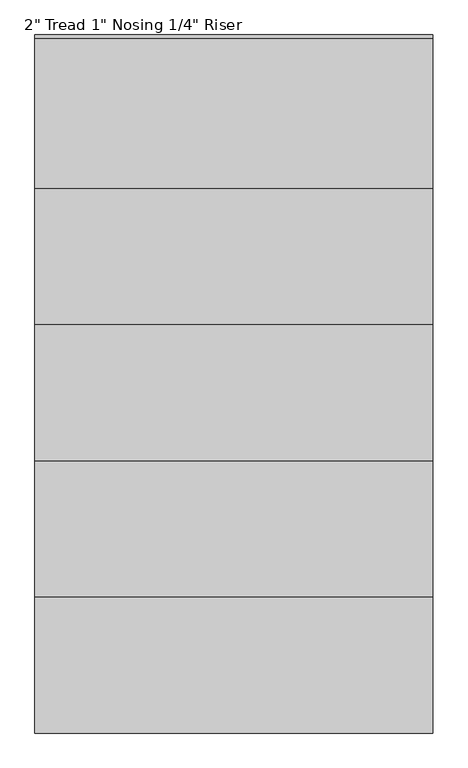
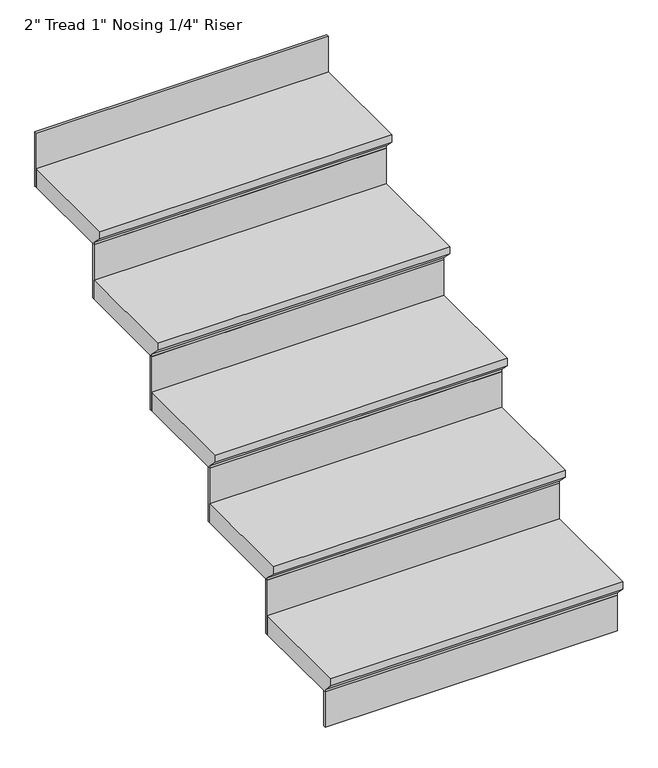
"""IFC4 building model written with IfcOpenShell, lengths in millimetres: stair flight geometry."""

from ifc_helpers import new_model, si_unit, origin, place, context, project, spatial, faceted_brep, source, transform, mapped, element, save


def stair_flight_3ae1c9df(model_context):
    return source(origin(), model_context, "Body", "Brep", [
        faceted_brep([(-5330.5155596, 4813.6076853, 127.0), (-5330.5155596, 4813.6076853, 146.05), (-6072.1955596, 4813.6076853, 146.05), (-6072.1955596, 4813.6076853, 127.0), (-5330.5155596, 4839.0076853, 101.6), (-6072.1955596, 4839.0076853, 101.6), (-5330.5155596, 5093.0076853, 146.05), (-6072.1955596, 5093.0076853, 146.05), (-6072.1955596, 4839.0076853, 95.25), (-6072.1955596, 5093.0076853, 95.25), (-5330.5155596, 5093.0076853, 95.25), (-5330.5155596, 4839.0076853, 95.25)], [[[0, 1, 2, 3]], [[4, 0, 3, 5]], [[2, 1, 6, 7]], [[8, 9, 10, 11]], [[2, 7, 9, 8, 5, 3]], [[8, 11, 4, 5]], [[6, 1, 0, 4, 11, 10]], [[7, 6, 10, 9]]]),
        faceted_brep([(-5330.5155596, 4839.0076853, 95.25), (-5330.5155596, 4839.0076853, 0.0), (-5330.5155596, 4845.3576853, 0.0), (-5330.5155596, 4845.3576853, 95.25), (-6072.1955596, 4839.0076853, 95.25), (-6072.1955596, 4845.3576853, 95.25), (-6072.1955596, 4845.3576853, 0.0), (-6072.1955596, 4839.0076853, 0.0)], [[[0, 1, 2, 3]], [[4, 5, 6, 7]], [[1, 0, 4, 7]], [[2, 1, 7, 6]], [[3, 2, 6, 5]], [[0, 3, 5, 4]]]),
        faceted_brep([(-5330.5155596, 5093.0076853, 241.3), (-5330.5155596, 5093.0076853, 95.25), (-5330.5155596, 5099.3576853, 95.25), (-5330.5155596, 5099.3576853, 241.3), (-6072.1955596, 5093.0076853, 241.3), (-6072.1955596, 5099.3576853, 241.3), (-6072.1955596, 5099.3576853, 95.25), (-6072.1955596, 5093.0076853, 95.25)], [[[0, 1, 2, 3]], [[4, 5, 6, 7]], [[1, 0, 4, 7]], [[2, 1, 7, 6]], [[3, 2, 6, 5]], [[0, 3, 5, 4]]]),
        faceted_brep([(-6072.1955596, 5067.6076853, 292.1), (-5330.5155596, 5067.6076853, 292.1), (-5330.5155596, 5347.0076853, 292.1), (-6072.1955596, 5347.0076853, 292.1), (-6072.1955596, 5093.0076853, 241.3), (-6072.1955596, 5347.0076853, 241.3), (-5330.5155596, 5347.0076853, 241.3), (-5330.5155596, 5093.0076853, 241.3), (-6072.1955596, 5093.0076853, 247.65), (-6072.1955596, 5067.6076853, 273.05), (-5330.5155596, 5093.0076853, 247.65), (-5330.5155596, 5067.6076853, 273.05)], [[[0, 1, 2, 3]], [[4, 5, 6, 7]], [[0, 3, 5, 4, 8, 9]], [[4, 7, 10, 8]], [[2, 1, 11, 10, 7, 6]], [[3, 2, 6, 5]], [[11, 1, 0, 9]], [[10, 11, 9, 8]]]),
        faceted_brep([(-5330.5155596, 5347.0076853, 387.35), (-5330.5155596, 5347.0076853, 241.3), (-5330.5155596, 5353.3576853, 241.3), (-5330.5155596, 5353.3576853, 387.35), (-6072.1955596, 5347.0076853, 387.35), (-6072.1955596, 5353.3576853, 387.35), (-6072.1955596, 5353.3576853, 241.3), (-6072.1955596, 5347.0076853, 241.3)], [[[0, 1, 2, 3]], [[4, 5, 6, 7]], [[1, 0, 4, 7]], [[2, 1, 7, 6]], [[3, 2, 6, 5]], [[0, 3, 5, 4]]]),
        faceted_brep([(-6072.1955596, 5321.6076853, 438.15), (-5330.5155596, 5321.6076853, 438.15), (-5330.5155596, 5601.0076853, 438.15), (-6072.1955596, 5601.0076853, 438.15), (-6072.1955596, 5347.0076853, 387.35), (-6072.1955596, 5601.0076853, 387.35), (-5330.5155596, 5601.0076853, 387.35), (-5330.5155596, 5347.0076853, 387.35), (-6072.1955596, 5347.0076853, 393.7), (-6072.1955596, 5321.6076853, 419.1), (-5330.5155596, 5347.0076853, 393.7), (-5330.5155596, 5321.6076853, 419.1)], [[[0, 1, 2, 3]], [[4, 5, 6, 7]], [[0, 3, 5, 4, 8, 9]], [[4, 7, 10, 8]], [[2, 1, 11, 10, 7, 6]], [[3, 2, 6, 5]], [[11, 1, 0, 9]], [[10, 11, 9, 8]]]),
        faceted_brep([(-5330.5155596, 5601.0076853, 533.4), (-5330.5155596, 5601.0076853, 387.35), (-5330.5155596, 5607.3576853, 387.35), (-5330.5155596, 5607.3576853, 533.4), (-6072.1955596, 5601.0076853, 533.4), (-6072.1955596, 5607.3576853, 533.4), (-6072.1955596, 5607.3576853, 387.35), (-6072.1955596, 5601.0076853, 387.35)], [[[0, 1, 2, 3]], [[4, 5, 6, 7]], [[1, 0, 4, 7]], [[2, 1, 7, 6]], [[3, 2, 6, 5]], [[0, 3, 5, 4]]]),
        faceted_brep([(-6072.1955596, 5575.6076853, 584.2), (-5330.5155596, 5575.6076853, 584.2), (-5330.5155596, 5855.0076853, 584.2), (-6072.1955596, 5855.0076853, 584.2), (-6072.1955596, 5601.0076853, 533.4), (-6072.1955596, 5855.0076853, 533.4), (-5330.5155596, 5855.0076853, 533.4), (-5330.5155596, 5601.0076853, 533.4), (-6072.1955596, 5601.0076853, 539.75), (-6072.1955596, 5575.6076853, 565.15), (-5330.5155596, 5601.0076853, 539.75), (-5330.5155596, 5575.6076853, 565.15)], [[[0, 1, 2, 3]], [[4, 5, 6, 7]], [[0, 3, 5, 4, 8, 9]], [[4, 7, 10, 8]], [[2, 1, 11, 10, 7, 6]], [[3, 2, 6, 5]], [[11, 1, 0, 9]], [[10, 11, 9, 8]]]),
        faceted_brep([(-5330.5155596, 6109.0076853, 825.5), (-5330.5155596, 6109.0076853, 679.45), (-5330.5155596, 6115.3576853, 679.45), (-5330.5155596, 6115.3576853, 825.5), (-6072.1955596, 6109.0076853, 825.5), (-6072.1955596, 6115.3576853, 825.5), (-6072.1955596, 6115.3576853, 679.45), (-6072.1955596, 6109.0076853, 679.45)], [[[0, 1, 2, 3]], [[4, 5, 6, 7]], [[1, 0, 4, 7]], [[2, 1, 7, 6]], [[3, 2, 6, 5]], [[0, 3, 5, 4]]]),
        faceted_brep([(-5330.5155596, 5855.0076853, 679.45), (-5330.5155596, 5855.0076853, 533.4), (-5330.5155596, 5861.3576853, 533.4), (-5330.5155596, 5861.3576853, 679.45), (-6072.1955596, 5855.0076853, 679.45), (-6072.1955596, 5861.3576853, 679.45), (-6072.1955596, 5861.3576853, 533.4), (-6072.1955596, 5855.0076853, 533.4)], [[[0, 1, 2, 3]], [[4, 5, 6, 7]], [[1, 0, 4, 7]], [[2, 1, 7, 6]], [[3, 2, 6, 5]], [[0, 3, 5, 4]]]),
        faceted_brep([(-6072.1955596, 5829.6076853, 730.25), (-5330.5155596, 5829.6076853, 730.25), (-5330.5155596, 6083.6076853, 730.25), (-5330.5155596, 6109.0076853, 730.25), (-6072.1955596, 6109.0076853, 730.25), (-6072.1955596, 5855.0076853, 679.45), (-6072.1955596, 6109.0076853, 679.45), (-5330.5155596, 6109.0076853, 679.45), (-5330.5155596, 6083.6076853, 679.45), (-5330.5155596, 5855.0076853, 679.45), (-6072.1955596, 5855.0076853, 685.8), (-6072.1955596, 5829.6076853, 711.2), (-5330.5155596, 5855.0076853, 685.8), (-5330.5155596, 5829.6076853, 711.2)], [[[0, 1, 2, 3, 4]], [[5, 6, 7, 8, 9]], [[0, 4, 6, 5, 10, 11]], [[5, 9, 12, 10]], [[2, 1, 13, 12, 9, 8]], [[3, 2, 8, 7]], [[4, 3, 7, 6]], [[13, 1, 0, 11]], [[12, 13, 11, 10]]]),
    ])


if __name__ == "__main__":
    model = new_model("IFC4")
    model_context = context("Model", 3, world=origin())
    ifc_project = project(units=[si_unit("LENGTHUNIT", "METRE", prefix="MILLI")], contexts=[model_context])
    site = spatial("IfcSite", under=ifc_project)
    building = spatial("IfcBuilding", under=site)
    placement = place(None, origin())
    stair_flight_shape = stair_flight_3ae1c9df(model_context)
    element("IfcStairFlight", 1, ObjectType="2\" Tread 1\" Nosing 1/4\" Riser", at=placement, inside=building, context=model_context, shape_type="MappedRepresentation", body=[
        mapped(stair_flight_shape, transform((0.0, 0.0, 0.0), x_axis=(1.0, 0.0, 0.0), y_axis=(0.0, 1.0, 0.0), z_axis=(0.0, 0.0, 1.0))),
    ])
    save(model, "model.ifc")
